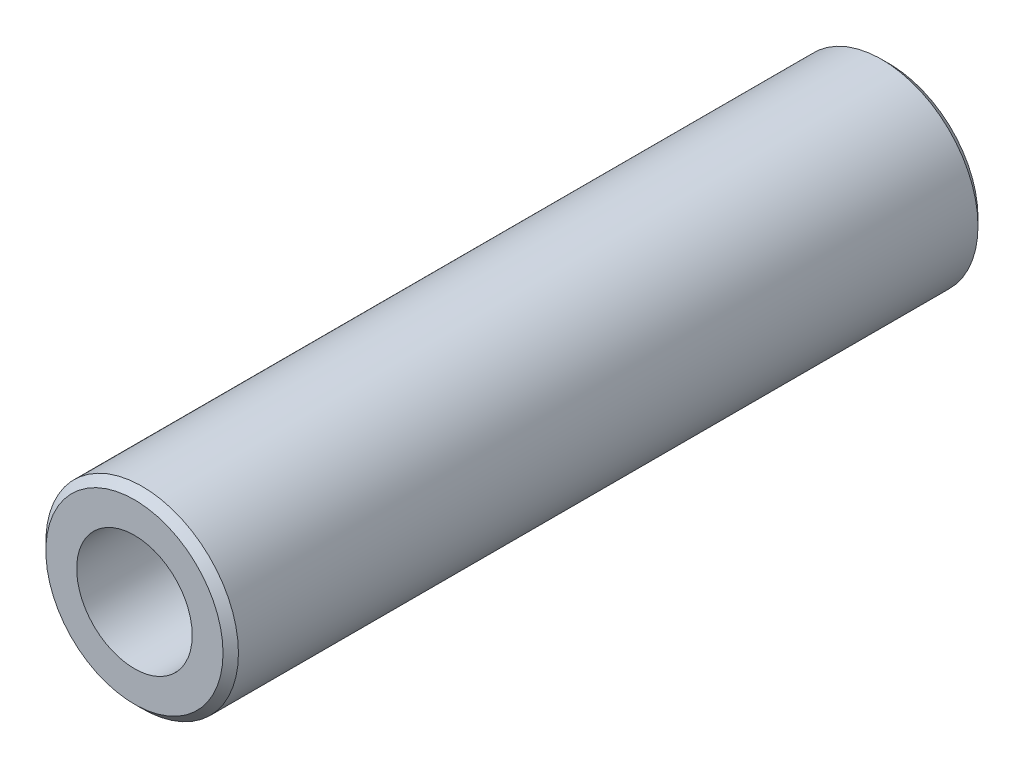
SolidWorks part; units mm, degrees
material "Plain Carbon Steel"
ref_plane "Front Plane" through (0, 0, 0) normal (0, 0, 1) x (1, 0, 0)
ref_plane "Top Plane" through (0, 0, 0) normal (0, 1, 0) x (1, 0, 0)
ref_plane "Right Plane" through (0, 0, 0) normal (1, 0, 0) x (0, 0, -1)
sketch "Pin OD Profile Ø12.5" plane through (0, 0, 0) normal (0, 0, 1) x (1, 0, 0)
  circle A0 centre (0, 0) radius 6.25
  dimension "D1" = 12.5
extrude "Pin Tube L49 Wall 2.5" add sketch "Pin OD Profile Ø12.5" along normal mid plane 49 thin thin type one direction reverse wall 2.5
chamfer "Pin Edge Chamfer 0.5x45°" distance 0.5 angle 45 2 edges at (6.25, 0, -24.5) (6.25, 0, 24.5)
